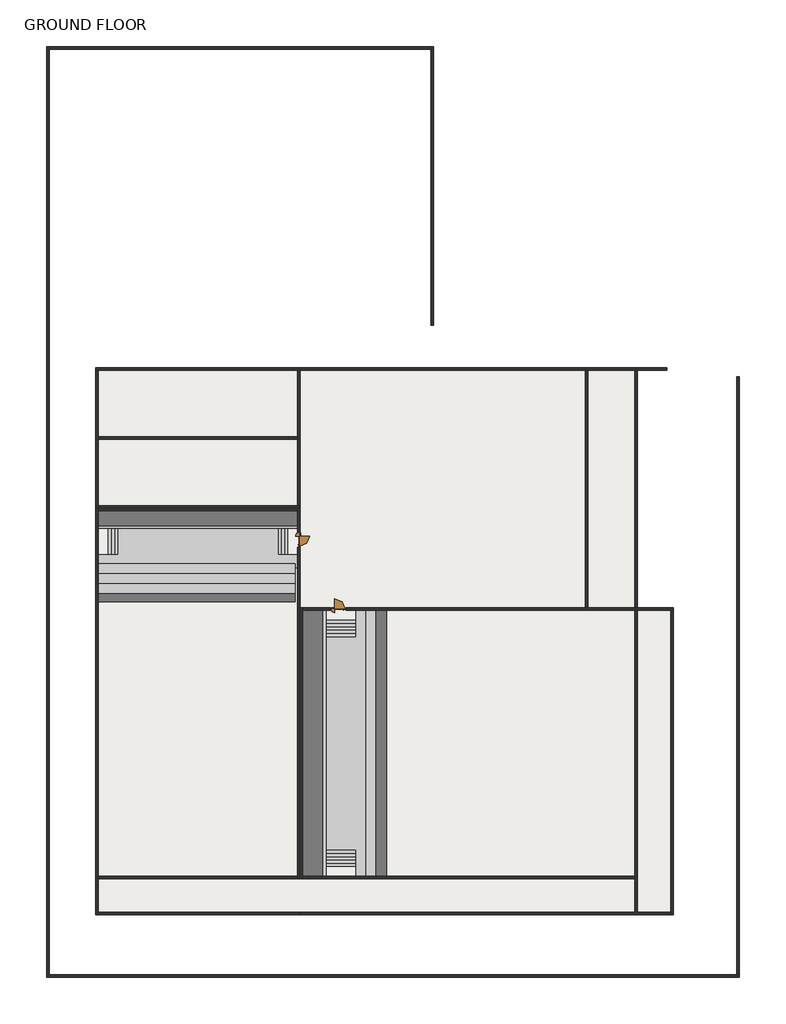
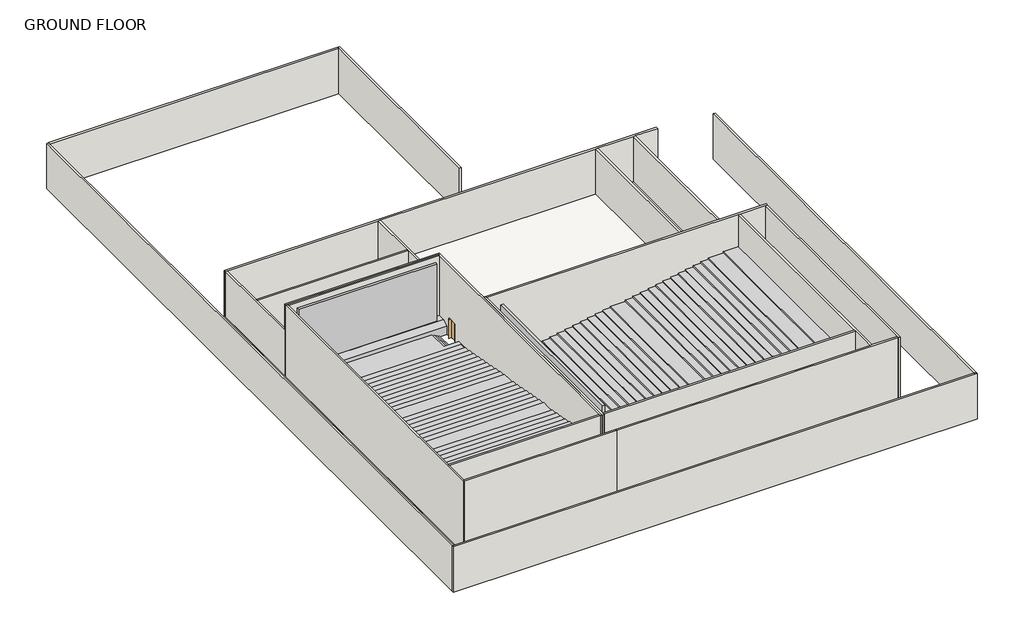
# One storey: 23 walls, 2 doors, 2 stair flights, 1 proxy, 1 slab.
"""IFC4 building model written with IfcOpenShell, lengths in millimetres."""

from ifc_helpers import new_model, si_unit, frame, origin, origin_with_axes, place, context, project, spatial, polyline, outline, extrude, faceted_brep, transform, mapped, element, save
from components import screen_1_screen_1_327eb079, door_1418x2438_e3a65d4f

model = new_model("IFC4")

# Units and contexts
model_context = context("Model", 3, world=origin())
ifc_project = project(units=[si_unit("LENGTHUNIT", "METRE", prefix="MILLI")], contexts=[model_context])

# Site, building, storey
site = spatial("IfcSite", under=ifc_project)
building = spatial("IfcBuilding", under=site)
storey = spatial("IfcBuildingStorey", under=building, Name="GROUND FLOOR", Elevation=0.0)

# Proxy
placement = place(None, origin())
screen_1_screen_1_shape = screen_1_screen_1_327eb079(model_context)
element("IfcBuildingElementProxy", 1, Name="SCREEN 1 : SCREEN 1", ObjectType="SCREEN 1 : SCREEN 1", at=placement, inside=storey, context=model_context, shape_type="MappedRepresentation", body=[
    mapped(screen_1_screen_1_shape, transform((0.0, 0.0, 0.0), x_axis=(1.0, 0.0, 0.0), y_axis=(0.0, 1.0, 0.0), z_axis=(0.0, 0.0, 1.0))),
])

# Doors
door_1418x2438_shape = door_1418x2438_e3a65d4f(model_context)
element("IfcDoor", 2, ObjectType="1418x2438", at=placement, inside=storey, context=model_context, shape_type="MappedRepresentation", body=[
    mapped(door_1418x2438_shape, transform((1375.3587563, 2839.4794445, 0.0), x_axis=(0.0, -1.0, 0.0), y_axis=(1.0, 0.0, 0.0), z_axis=(0.0, 0.0, 1.0))),
])
element("IfcDoor", 3, ObjectType="1418x2438", at=placement, inside=storey, context=model_context, shape_type="MappedRepresentation", body=[
    mapped(door_1418x2438_shape, transform((4956.7587563, -3561.3205555, 0.0), x_axis=(1.0, 0.0, 0.0), y_axis=(0.0, 1.0, 0.0), z_axis=(0.0, 0.0, 1.0))),
])

# Slab
element("IfcSlab", 4, ObjectType="screen room floor 1'", at=placement, inside=storey, context=model_context, shape_type="SweptSolid", body=[
    extrude(outline(polyline([(32426.8587563, 18574.7794445), (32426.8587563, -3447.0205555), (35703.4587563, -3447.0205555), (35703.4587563, -31564.8205555), (-17255.5412437, -31564.8205555), (-17255.5412437, 18574.7794445), (32426.8587563, 18574.7794445)])), frame((0.0, 0.0, -304.8), z_axis=(0.0, 0.0, 1.0), x_axis=(1.0, 0.0, 0.0)), (0.0, 0.0, 1.0), 304.8),
])

# Stair flights
element("IfcStairFlight", 5, ObjectType="3/4\" Nosing", at=placement, inside=storey, context=model_context, shape_type="Brep", body=[
    faceted_brep([(1032.4587563, -322.8205555, 782.5678049), (1032.4587563, 591.5794445, 782.5678049), (-17026.9412437, 591.5794445, 782.5678049), (-17026.9412437, -322.8205555, 782.5678049), (1032.4587563, -322.8205555, 717.941728), (1032.4587563, 249.9315597, 609.6), (1032.4587563, 591.5794445, 609.6), (-17026.9412437, 591.5794445, 609.6), (-17026.9412437, 249.9315597, 609.6), (-17026.9412437, -322.8205555, 717.941728), (1032.4587563, -1237.2205555, 955.5356098), (1032.4587563, -322.8205555, 955.5356098), (-17026.9412437, -322.8205555, 955.5356098), (-17026.9412437, -1237.2205555, 955.5356098), (1032.4587563, -1237.2205555, 890.9095329), (-17026.9412437, -1237.2205555, 890.9095329), (1032.4587563, -2151.6205555, 1128.5034146), (1032.4587563, -1237.2205555, 1128.5034146), (-17026.9412437, -1237.2205555, 1128.5034146), (-17026.9412437, -2151.6205555, 1128.5034146), (1032.4587563, -2151.6205555, 1063.8773378), (-17026.9412437, -2151.6205555, 1063.8773378), (1032.4587563, -3066.0205555, 1301.4712195), (1032.4587563, -2151.6205555, 1301.4712195), (-17026.9412437, -2151.6205555, 1301.4712195), (-17026.9412437, -3066.0205555, 1301.4712195), (1032.4587563, -3066.0205555, 1236.8451427), (-17026.9412437, -3066.0205555, 1236.8451427), (1032.4587563, -3980.4205555, 1474.4390244), (1032.4587563, -3066.0205555, 1474.4390244), (-17026.9412437, -3066.0205555, 1474.4390244), (-17026.9412437, -3980.4205555, 1474.4390244), (1032.4587563, -3980.4205555, 1409.8129475), (-17026.9412437, -3980.4205555, 1409.8129475), (1032.4587563, -4894.8205555, 1647.4068293), (1032.4587563, -3980.4205555, 1647.4068293), (-17026.9412437, -3980.4205555, 1647.4068293), (-17026.9412437, -4894.8205555, 1647.4068293), (1032.4587563, -4894.8205555, 1582.7807524), (-17026.9412437, -4894.8205555, 1582.7807524), (1032.4587563, -5809.2205555, 1820.3746341), (1032.4587563, -4894.8205555, 1820.3746341), (-17026.9412437, -4894.8205555, 1820.3746341), (-17026.9412437, -5809.2205555, 1820.3746341), (1032.4587563, -5809.2205555, 1755.7485573), (-17026.9412437, -5809.2205555, 1755.7485573), (1032.4587563, -6723.6205555, 1993.342439), (1032.4587563, -5809.2205555, 1993.342439), (-17026.9412437, -5809.2205555, 1993.342439), (-17026.9412437, -6723.6205555, 1993.342439), (1032.4587563, -6723.6205555, 1928.7163622), (-17026.9412437, -6723.6205555, 1928.7163622), (1032.4587563, -7638.0205555, 2166.3102439), (1032.4587563, -6723.6205555, 2166.3102439), (-17026.9412437, -6723.6205555, 2166.3102439), (-17026.9412437, -7638.0205555, 2166.3102439), (1032.4587563, -7638.0205555, 2101.684167), (-17026.9412437, -7638.0205555, 2101.684167), (1032.4587563, -8552.4205555, 2512.2458537), (-17026.9412437, -8552.4205555, 2512.2458537), (-17026.9412437, -9472.7735979, 2512.2458537), (-17026.9412437, -10381.2205555, 2512.2458537), (1032.4587563, -10381.2205555, 2512.2458537), (1032.4587563, -9472.7735979, 2512.2458537), (1032.4587563, -8552.4205555, 2339.2780488), (1032.4587563, -10381.2205555, 2448.7458537), (1032.4587563, -9472.7735979, 2448.7458537), (1032.4587563, -8552.4205555, 2274.6519719), (-17026.9412437, -8552.4205555, 2339.2780488), (-17026.9412437, -8552.4205555, 2274.6519719), (-17026.9412437, -9472.7735979, 2448.7458537), (-17026.9412437, -10381.2205555, 2448.7458537), (1032.4587563, -18610.8205555, 4068.9560976), (-17026.9412437, -18610.8205555, 4068.9560976), (-17026.9412437, -18616.7735979, 4068.9560976), (-17026.9412437, -19525.2205555, 4068.9560976), (1032.4587563, -19525.2205555, 4068.9560976), (1032.4587563, -18616.7735979, 4068.9560976), (1032.4587563, -18610.8205555, 3895.9882927), (1032.4587563, -19525.2205555, 4004.3300207), (1032.4587563, -18616.7735979, 3832.4882927), (1032.4587563, -18610.8205555, 3832.4882927), (-17026.9412437, -18610.8205555, 3895.9882927), (-17026.9412437, -18610.8205555, 3832.4882927), (-17026.9412437, -18616.7735979, 3832.4882927), (-17026.9412437, -19525.2205555, 4004.3300207), (1032.4587563, -10387.1735979, 2448.7458537), (-17026.9412437, -10387.1735979, 2448.7458537), (1032.4587563, -11295.6205555, 2620.5875817), (1032.4587563, -12210.0205555, 2793.5553866), (1032.4587563, -13124.4205555, 2966.5231914), (1032.4587563, -14038.8205555, 3139.4909963), (1032.4587563, -14953.2205555, 3312.4588012), (1032.4587563, -15867.6205555, 3485.4266061), (1032.4587563, -16782.0205555, 3658.3944109), (1032.4587563, -17702.3735979, 3832.4882927), (-17026.9412437, -17702.3735979, 3832.4882927), (-17026.9412437, -16782.0205555, 3658.3944109), (-17026.9412437, -15867.6205555, 3485.4266061), (-17026.9412437, -14953.2205555, 3312.4588012), (-17026.9412437, -14038.8205555, 3139.4909963), (-17026.9412437, -13124.4205555, 2966.5231914), (-17026.9412437, -12210.0205555, 2793.5553866), (-17026.9412437, -11295.6205555, 2620.5875817), (1032.4587563, -20439.6205555, 4177.2978256), (1032.4587563, -21354.0205555, 4350.2656305), (1032.4587563, -22268.4205555, 4523.2334353), (1032.4587563, -23182.8205555, 4696.2012402), (1032.4587563, -24097.2205555, 4869.1690451), (1032.4587563, -25011.6205555, 5042.13685), (1032.4587563, -25926.0205555, 5215.1046548), (1032.4587563, -26840.4205555, 5388.0724597), (1032.4587563, -27760.7735979, 5562.1663415), (-17026.9412437, -27760.7735979, 5562.1663415), (-17026.9412437, -26840.4205555, 5388.0724597), (-17026.9412437, -25926.0205555, 5215.1046548), (-17026.9412437, -25011.6205555, 5042.13685), (-17026.9412437, -24097.2205555, 4869.1690451), (-17026.9412437, -23182.8205555, 4696.2012402), (-17026.9412437, -22268.4205555, 4523.2334353), (-17026.9412437, -21354.0205555, 4350.2656305), (-17026.9412437, -20439.6205555, 4177.2978256), (1032.4587563, -7638.0205555, 2339.2780488), (-17026.9412437, -7638.0205555, 2339.2780488), (1032.4587563, -10381.2205555, 2685.2136585), (-17026.9412437, -10381.2205555, 2685.2136585), (-17026.9412437, -10387.1735979, 2685.2136585), (-17026.9412437, -11295.6205555, 2685.2136585), (1032.4587563, -11295.6205555, 2685.2136585), (1032.4587563, -10387.1735979, 2685.2136585), (1032.4587563, -12210.0205555, 2858.1814634), (1032.4587563, -11295.6205555, 2858.1814634), (-17026.9412437, -11295.6205555, 2858.1814634), (-17026.9412437, -12210.0205555, 2858.1814634), (1032.4587563, -13124.4205555, 3031.1492683), (1032.4587563, -12210.0205555, 3031.1492683), (-17026.9412437, -12210.0205555, 3031.1492683), (-17026.9412437, -13124.4205555, 3031.1492683), (1032.4587563, -14038.8205555, 3204.1170732), (1032.4587563, -13124.4205555, 3204.1170732), (-17026.9412437, -13124.4205555, 3204.1170732), (-17026.9412437, -14038.8205555, 3204.1170732), (1032.4587563, -14953.2205555, 3377.084878), (1032.4587563, -14038.8205555, 3377.084878), (-17026.9412437, -14038.8205555, 3377.084878), (-17026.9412437, -14953.2205555, 3377.084878), (1032.4587563, -15867.6205555, 3550.0526829), (1032.4587563, -14953.2205555, 3550.0526829), (-17026.9412437, -14953.2205555, 3550.0526829), (-17026.9412437, -15867.6205555, 3550.0526829), (1032.4587563, -16782.0205555, 3723.0204878), (1032.4587563, -15867.6205555, 3723.0204878), (-17026.9412437, -15867.6205555, 3723.0204878), (-17026.9412437, -16782.0205555, 3723.0204878), (1032.4587563, -16782.0205555, 3895.9882927), (-17026.9412437, -16782.0205555, 3895.9882927), (-17026.9412437, -17702.3735979, 3895.9882927), (1032.4587563, -17702.3735979, 3895.9882927), (1032.4587563, -20439.6205555, 4241.9239024), (1032.4587563, -19525.2205555, 4241.9239024), (-17026.9412437, -19525.2205555, 4241.9239024), (-17026.9412437, -20439.6205555, 4241.9239024), (1032.4587563, -21354.0205555, 4414.8917073), (1032.4587563, -20439.6205555, 4414.8917073), (-17026.9412437, -20439.6205555, 4414.8917073), (-17026.9412437, -21354.0205555, 4414.8917073), (1032.4587563, -22268.4205555, 4587.8595122), (1032.4587563, -21354.0205555, 4587.8595122), (-17026.9412437, -21354.0205555, 4587.8595122), (-17026.9412437, -22268.4205555, 4587.8595122), (1032.4587563, -23182.8205555, 4760.8273171), (1032.4587563, -22268.4205555, 4760.8273171), (-17026.9412437, -22268.4205555, 4760.8273171), (-17026.9412437, -23182.8205555, 4760.8273171), (1032.4587563, -24097.2205555, 4933.795122), (1032.4587563, -23182.8205555, 4933.795122), (-17026.9412437, -23182.8205555, 4933.795122), (-17026.9412437, -24097.2205555, 4933.795122), (1032.4587563, -25011.6205555, 5106.7629268), (1032.4587563, -24097.2205555, 5106.7629268), (-17026.9412437, -24097.2205555, 5106.7629268), (-17026.9412437, -25011.6205555, 5106.7629268), (1032.4587563, -25926.0205555, 5279.7307317), (1032.4587563, -25011.6205555, 5279.7307317), (-17026.9412437, -25011.6205555, 5279.7307317), (-17026.9412437, -25926.0205555, 5279.7307317), (1032.4587563, -26840.4205555, 5452.6985366), (1032.4587563, -25926.0205555, 5452.6985366), (-17026.9412437, -25926.0205555, 5452.6985366), (-17026.9412437, -26840.4205555, 5452.6985366), (1032.4587563, -26840.4205555, 5625.6663415), (-17026.9412437, -26840.4205555, 5625.6663415), (-17026.9412437, -27760.7735979, 5625.6663415), (-17026.9412437, -28059.6205555, 5625.6663415), (1032.4587563, -28059.6205555, 5625.6663415), (1032.4587563, -27760.7735979, 5625.6663415), (1032.4587563, -28059.6205555, 5562.1663415), (-17026.9412437, -28059.6205555, 5562.1663415)], [[[0, 1, 2, 3]], [[1, 0, 4, 5, 6]], [[2, 1, 6, 7]], [[3, 2, 7, 8, 9]], [[10, 11, 12, 13]], [[11, 10, 14, 4, 0]], [[0, 3, 12, 11]], [[13, 12, 3, 9, 15]], [[16, 17, 18, 19]], [[17, 16, 20, 14, 10]], [[10, 13, 18, 17]], [[19, 18, 13, 15, 21]], [[22, 23, 24, 25]], [[23, 22, 26, 20, 16]], [[16, 19, 24, 23]], [[25, 24, 19, 21, 27]], [[28, 29, 30, 31]], [[29, 28, 32, 26, 22]], [[22, 25, 30, 29]], [[31, 30, 25, 27, 33]], [[34, 35, 36, 37]], [[35, 34, 38, 32, 28]], [[28, 31, 36, 35]], [[37, 36, 31, 33, 39]], [[40, 41, 42, 43]], [[41, 40, 44, 38, 34]], [[34, 37, 42, 41]], [[43, 42, 37, 39, 45]], [[46, 47, 48, 49]], [[47, 46, 50, 44, 40]], [[40, 43, 48, 47]], [[49, 48, 43, 45, 51]], [[52, 53, 54, 55]], [[53, 52, 56, 50, 46]], [[46, 49, 54, 53]], [[55, 54, 49, 51, 57]], [[58, 59, 60, 61, 62, 63]], [[64, 58, 63, 62, 65, 66, 67]], [[64, 68, 59, 58]], [[59, 68, 69, 70, 71, 61, 60]], [[72, 73, 74, 75, 76, 77]], [[78, 72, 77, 76, 79, 80, 81]], [[78, 82, 73, 72]], [[73, 82, 83, 84, 85, 75, 74]], [[7, 6, 5, 8]], [[66, 70, 69, 57, 51, 45, 39, 33, 27, 21, 15, 9, 8, 5, 4, 14, 20, 26, 32, 38, 44, 50, 56, 67]], [[70, 66, 65, 86, 87, 71]], [[87, 86, 88, 89, 90, 91, 92, 93, 94, 95, 96, 97, 98, 99, 100, 101, 102, 103]], [[96, 95, 81, 80, 84, 83]], [[84, 80, 79, 104, 105, 106, 107, 108, 109, 110, 111, 112, 113, 114, 115, 116, 117, 118, 119, 120, 121, 85]], [[64, 122, 123, 68]], [[122, 64, 67, 56, 52]], [[52, 55, 123, 122]], [[68, 123, 55, 57, 69]], [[124, 125, 126, 127, 128, 129]], [[62, 124, 129, 128, 88, 86, 65]], [[62, 61, 125, 124]], [[125, 61, 71, 87, 103, 127, 126]], [[130, 131, 132, 133]], [[131, 130, 89, 88, 128]], [[128, 127, 132, 131]], [[133, 132, 127, 103, 102]], [[134, 135, 136, 137]], [[135, 134, 90, 89, 130]], [[130, 133, 136, 135]], [[137, 136, 133, 102, 101]], [[138, 139, 140, 141]], [[139, 138, 91, 90, 134]], [[134, 137, 140, 139]], [[141, 140, 137, 101, 100]], [[142, 143, 144, 145]], [[143, 142, 92, 91, 138]], [[138, 141, 144, 143]], [[145, 144, 141, 100, 99]], [[146, 147, 148, 149]], [[147, 146, 93, 92, 142]], [[142, 145, 148, 147]], [[149, 148, 145, 99, 98]], [[150, 151, 152, 153]], [[151, 150, 94, 93, 146]], [[146, 149, 152, 151]], [[153, 152, 149, 98, 97]], [[154, 155, 156, 82, 78, 157]], [[150, 154, 157, 78, 81, 95, 94]], [[150, 153, 155, 154]], [[155, 153, 97, 96, 83, 82, 156]], [[158, 159, 160, 161]], [[159, 158, 104, 79, 76]], [[76, 75, 160, 159]], [[161, 160, 75, 85, 121]], [[162, 163, 164, 165]], [[163, 162, 105, 104, 158]], [[158, 161, 164, 163]], [[165, 164, 161, 121, 120]], [[166, 167, 168, 169]], [[167, 166, 106, 105, 162]], [[162, 165, 168, 167]], [[169, 168, 165, 120, 119]], [[170, 171, 172, 173]], [[171, 170, 107, 106, 166]], [[166, 169, 172, 171]], [[173, 172, 169, 119, 118]], [[174, 175, 176, 177]], [[175, 174, 108, 107, 170]], [[170, 173, 176, 175]], [[177, 176, 173, 118, 117]], [[178, 179, 180, 181]], [[179, 178, 109, 108, 174]], [[174, 177, 180, 179]], [[181, 180, 177, 117, 116]], [[182, 183, 184, 185]], [[183, 182, 110, 109, 178]], [[178, 181, 184, 183]], [[185, 184, 181, 116, 115]], [[186, 187, 188, 189]], [[187, 186, 111, 110, 182]], [[182, 185, 188, 187]], [[189, 188, 185, 115, 114]], [[190, 191, 192, 193, 194, 195]], [[186, 190, 195, 194, 196, 112, 111]], [[186, 189, 191, 190]], [[191, 189, 114, 113, 197, 193, 192]], [[194, 193, 197, 196]], [[113, 112, 196, 197]]]),
])
element("IfcStairFlight", 6, ObjectType="3/4\" Nosing", at=placement, inside=storey, context=model_context, shape_type="Brep", body=[
    faceted_brep([(8423.8587563, -3675.6205555, 1085.3853659), (7509.4587563, -3675.6205555, 1085.3853659), (7509.4587563, -28059.6205555, 1085.3853659), (8423.8587563, -28059.6205555, 1085.3853659), (8423.8587563, -3675.6205555, 1020.7847351), (7854.9316945, -3675.6205555, 914.4), (7509.4587563, -3675.6205555, 914.4), (7509.4587563, -28059.6205555, 914.4), (7854.9316945, -28059.6205555, 914.4), (8423.8587563, -28059.6205555, 1020.7847351), (9338.2587563, -3675.6205555, 1256.3707317), (8423.8587563, -3675.6205555, 1256.3707317), (8423.8587563, -28059.6205555, 1256.3707317), (9338.2587563, -28059.6205555, 1256.3707317), (9338.2587563, -3675.6205555, 1191.770101), (9338.2587563, -28059.6205555, 1191.770101), (10252.6587563, -3675.6205555, 1427.3560976), (9338.2587563, -3675.6205555, 1427.3560976), (9338.2587563, -28059.6205555, 1427.3560976), (10252.6587563, -28059.6205555, 1427.3560976), (10252.6587563, -3675.6205555, 1362.7554668), (10252.6587563, -28059.6205555, 1362.7554668), (11167.0587563, -3675.6205555, 1598.3414634), (10252.6587563, -3675.6205555, 1598.3414634), (10252.6587563, -28059.6205555, 1598.3414634), (11167.0587563, -28059.6205555, 1598.3414634), (11167.0587563, -3675.6205555, 1533.7408327), (11167.0587563, -28059.6205555, 1533.7408327), (12081.4587563, -3675.6205555, 1769.3268293), (11167.0587563, -3675.6205555, 1769.3268293), (11167.0587563, -28059.6205555, 1769.3268293), (12081.4587563, -28059.6205555, 1769.3268293), (12081.4587563, -3675.6205555, 1704.7261985), (12081.4587563, -28059.6205555, 1704.7261985), (12995.8587563, -3675.6205555, 1940.3121951), (12081.4587563, -3675.6205555, 1940.3121951), (12081.4587563, -28059.6205555, 1940.3121951), (12995.8587563, -28059.6205555, 1940.3121951), (12995.8587563, -3675.6205555, 1875.7115644), (12995.8587563, -28059.6205555, 1875.7115644), (13910.2587563, -3675.6205555, 2111.297561), (12995.8587563, -3675.6205555, 2111.297561), (12995.8587563, -28059.6205555, 2111.297561), (13910.2587563, -28059.6205555, 2111.297561), (13910.2587563, -3675.6205555, 2046.6969303), (13910.2587563, -28059.6205555, 2046.6969303), (14824.6587563, -3675.6205555, 2282.2829268), (13910.2587563, -3675.6205555, 2282.2829268), (13910.2587563, -28059.6205555, 2282.2829268), (14824.6587563, -28059.6205555, 2282.2829268), (14824.6587563, -3675.6205555, 2217.6822961), (14824.6587563, -28059.6205555, 2217.6822961), (15739.0587563, -3675.6205555, 2453.2682927), (14824.6587563, -3675.6205555, 2453.2682927), (14824.6587563, -28059.6205555, 2453.2682927), (15739.0587563, -28059.6205555, 2453.2682927), (15739.0587563, -3675.6205555, 2388.667662), (15739.0587563, -28059.6205555, 2388.667662), (16653.4587563, -3675.6205555, 2624.2536585), (15739.0587563, -3675.6205555, 2624.2536585), (15739.0587563, -28059.6205555, 2624.2536585), (16653.4587563, -28059.6205555, 2624.2536585), (16653.4587563, -3675.6205555, 2559.6530278), (16653.4587563, -28059.6205555, 2559.6530278), (16653.4587563, -3675.6205555, 2795.2390244), (16653.4587563, -28059.6205555, 2795.2390244), (17573.7447379, -28059.6205555, 2795.2390244), (18482.2587563, -28059.6205555, 2795.2390244), (18482.2587563, -3675.6205555, 2795.2390244), (17573.7447379, -3675.6205555, 2795.2390244), (18482.2587563, -3675.6205555, 2731.7390244), (17573.7447379, -3675.6205555, 2731.7390244), (17573.7447379, -28059.6205555, 2731.7390244), (18482.2587563, -28059.6205555, 2731.7390244), (18482.2587563, -3675.6205555, 2966.2243902), (18482.2587563, -28059.6205555, 2966.2243902), (18488.1447379, -28059.6205555, 2966.2243902), (19396.6587563, -28059.6205555, 2966.2243902), (19396.6587563, -3675.6205555, 2966.2243902), (18488.1447379, -3675.6205555, 2966.2243902), (19396.6587563, -3675.6205555, 2901.6237595), (18488.1447379, -3675.6205555, 2731.7390244), (18488.1447379, -28059.6205555, 2731.7390244), (19396.6587563, -28059.6205555, 2901.6237595), (20311.0587563, -3675.6205555, 3137.2097561), (19396.6587563, -3675.6205555, 3137.2097561), (19396.6587563, -28059.6205555, 3137.2097561), (20311.0587563, -28059.6205555, 3137.2097561), (20311.0587563, -3675.6205555, 3072.6091254), (20311.0587563, -28059.6205555, 3072.6091254), (21225.4587563, -3675.6205555, 3308.195122), (20311.0587563, -3675.6205555, 3308.195122), (20311.0587563, -28059.6205555, 3308.195122), (21225.4587563, -28059.6205555, 3308.195122), (21225.4587563, -3675.6205555, 3243.5944912), (21225.4587563, -28059.6205555, 3243.5944912), (22139.8587563, -3675.6205555, 3479.1804878), (21225.4587563, -3675.6205555, 3479.1804878), (21225.4587563, -28059.6205555, 3479.1804878), (22139.8587563, -28059.6205555, 3479.1804878), (22139.8587563, -3675.6205555, 3414.5798571), (22139.8587563, -28059.6205555, 3414.5798571), (23054.2587563, -3675.6205555, 3650.1658537), (22139.8587563, -3675.6205555, 3650.1658537), (22139.8587563, -28059.6205555, 3650.1658537), (23054.2587563, -28059.6205555, 3650.1658537), (23054.2587563, -3675.6205555, 3585.5652229), (23054.2587563, -28059.6205555, 3585.5652229), (23968.6587563, -3675.6205555, 3821.1512195), (23054.2587563, -3675.6205555, 3821.1512195), (23054.2587563, -28059.6205555, 3821.1512195), (23968.6587563, -28059.6205555, 3821.1512195), (23968.6587563, -3675.6205555, 3756.5505888), (23968.6587563, -28059.6205555, 3756.5505888), (24883.0587563, -3675.6205555, 3992.1365854), (23968.6587563, -3675.6205555, 3992.1365854), (23968.6587563, -28059.6205555, 3992.1365854), (24883.0587563, -28059.6205555, 3992.1365854), (24883.0587563, -3675.6205555, 3927.5359546), (24883.0587563, -28059.6205555, 3927.5359546), (25797.4587563, -3675.6205555, 4163.1219512), (24883.0587563, -3675.6205555, 4163.1219512), (24883.0587563, -28059.6205555, 4163.1219512), (25797.4587563, -28059.6205555, 4163.1219512), (25797.4587563, -3675.6205555, 4098.5213205), (25797.4587563, -28059.6205555, 4098.5213205), (26711.8587563, -3675.6205555, 4334.1073171), (25797.4587563, -3675.6205555, 4334.1073171), (25797.4587563, -28059.6205555, 4334.1073171), (26711.8587563, -28059.6205555, 4334.1073171), (26711.8587563, -3675.6205555, 4269.5066863), (26711.8587563, -28059.6205555, 4269.5066863), (27626.2587563, -3675.6205555, 4505.0926829), (26711.8587563, -3675.6205555, 4505.0926829), (26711.8587563, -28059.6205555, 4505.0926829), (27626.2587563, -28059.6205555, 4505.0926829), (27626.2587563, -3675.6205555, 4440.4920522), (27626.2587563, -28059.6205555, 4440.4920522), (28540.6587563, -3675.6205555, 4676.0780488), (27626.2587563, -3675.6205555, 4676.0780488), (27626.2587563, -28059.6205555, 4676.0780488), (28540.6587563, -28059.6205555, 4676.0780488), (28540.6587563, -3675.6205555, 4612.3011104), (28540.6587563, -3675.6205555, 4611.4774181), (28540.6587563, -28059.6205555, 4611.4774181), (28540.6587563, -28059.6205555, 4612.3011104), (30369.4587563, -3675.6205555, 4847.0634146), (28540.6587563, -3675.6205555, 4847.0634146), (28540.6587563, -28059.6205555, 4847.0634146), (30369.4587563, -28059.6205555, 4847.0634146), (30369.4587563, -3675.6205555, 4783.2864762), (30369.4587563, -28059.6205555, 4783.2864762), (32198.2587563, -3675.6205555, 4954.2718421), (32198.2587563, -28059.6205555, 4954.2718421), (32198.2587563, -3675.6205555, 5018.0487805), (30369.4587563, -3675.6205555, 5018.0487805), (30369.4587563, -28059.6205555, 5018.0487805), (32198.2587563, -28059.6205555, 5018.0487805)], [[[0, 1, 2, 3]], [[1, 0, 4, 5, 6]], [[2, 1, 6, 7]], [[3, 2, 7, 8, 9]], [[10, 11, 12, 13]], [[11, 10, 14, 4, 0]], [[0, 3, 12, 11]], [[13, 12, 3, 9, 15]], [[16, 17, 18, 19]], [[17, 16, 20, 14, 10]], [[10, 13, 18, 17]], [[19, 18, 13, 15, 21]], [[22, 23, 24, 25]], [[23, 22, 26, 20, 16]], [[16, 19, 24, 23]], [[25, 24, 19, 21, 27]], [[28, 29, 30, 31]], [[29, 28, 32, 26, 22]], [[22, 25, 30, 29]], [[31, 30, 25, 27, 33]], [[34, 35, 36, 37]], [[35, 34, 38, 32, 28]], [[28, 31, 36, 35]], [[37, 36, 31, 33, 39]], [[40, 41, 42, 43]], [[41, 40, 44, 38, 34]], [[34, 37, 42, 41]], [[43, 42, 37, 39, 45]], [[46, 47, 48, 49]], [[47, 46, 50, 44, 40]], [[40, 43, 48, 47]], [[49, 48, 43, 45, 51]], [[52, 53, 54, 55]], [[53, 52, 56, 50, 46]], [[46, 49, 54, 53]], [[55, 54, 49, 51, 57]], [[58, 59, 60, 61]], [[59, 58, 62, 56, 52]], [[52, 55, 60, 59]], [[61, 60, 55, 57, 63]], [[64, 65, 66, 67, 68, 69]], [[58, 64, 69, 68, 70, 71, 62]], [[58, 61, 65, 64]], [[65, 61, 63, 72, 73, 67, 66]], [[74, 75, 76, 77, 78, 79]], [[68, 74, 79, 78, 80, 81, 70]], [[68, 67, 75, 74]], [[75, 67, 73, 82, 83, 77, 76]], [[84, 85, 86, 87]], [[85, 84, 88, 80, 78]], [[78, 77, 86, 85]], [[87, 86, 77, 83, 89]], [[90, 91, 92, 93]], [[91, 90, 94, 88, 84]], [[84, 87, 92, 91]], [[93, 92, 87, 89, 95]], [[96, 97, 98, 99]], [[97, 96, 100, 94, 90]], [[90, 93, 98, 97]], [[99, 98, 93, 95, 101]], [[102, 103, 104, 105]], [[103, 102, 106, 100, 96]], [[96, 99, 104, 103]], [[105, 104, 99, 101, 107]], [[108, 109, 110, 111]], [[109, 108, 112, 106, 102]], [[102, 105, 110, 109]], [[111, 110, 105, 107, 113]], [[114, 115, 116, 117]], [[115, 114, 118, 112, 108]], [[108, 111, 116, 115]], [[117, 116, 111, 113, 119]], [[120, 121, 122, 123]], [[121, 120, 124, 118, 114]], [[114, 117, 122, 121]], [[123, 122, 117, 119, 125]], [[126, 127, 128, 129]], [[127, 126, 130, 124, 120]], [[120, 123, 128, 127]], [[129, 128, 123, 125, 131]], [[132, 133, 134, 135]], [[133, 132, 136, 130, 126]], [[126, 129, 134, 133]], [[135, 134, 129, 131, 137]], [[138, 139, 140, 141]], [[139, 138, 142, 143, 136, 132]], [[132, 135, 140, 139]], [[141, 140, 135, 137, 144, 145]], [[146, 147, 148, 149]], [[147, 146, 150, 142, 138]], [[138, 141, 148, 147]], [[149, 148, 141, 145, 151]], [[7, 6, 5, 8]], [[71, 72, 63, 57, 51, 45, 39, 33, 27, 21, 15, 9, 8, 5, 4, 14, 20, 26, 32, 38, 44, 50, 56, 62]], [[72, 71, 70, 81, 82, 73]], [[143, 144, 137, 131, 125, 119, 113, 107, 101, 95, 89, 83, 82, 81, 80, 88, 94, 100, 106, 112, 118, 124, 130, 136]], [[144, 143, 142, 145]], [[145, 142, 150, 152, 153, 151]], [[154, 155, 156, 157]], [[155, 154, 152, 150, 146]], [[146, 149, 156, 155]], [[157, 156, 149, 151, 153]], [[154, 157, 153, 152]]]),
])

# Walls
element("IfcWall", 7, ObjectType="9\" inch wall", at=placement, inside=storey, context=model_context, shape_type="Brep", body=[
    faceted_brep([(-17255.5412437, 5696.9794445, 9144.0), (-17255.5412437, 5696.9794445, 0.0), (-17255.5412437, -31564.8205555, 0.0), (-17255.5412437, -31564.8205555, 9144.0), (-17026.9412437, 5696.9794445, 0.0), (-17026.9412437, 5696.9794445, 9144.0), (-17026.9412437, 5468.3794445, 9144.0), (-17026.9412437, -28059.6205555, 9144.0), (-17026.9412437, -28288.2205555, 9144.0), (-17026.9412437, -31336.2205555, 9144.0), (-17026.9412437, -31564.8205555, 9144.0), (-17026.9412437, -31564.8205555, 0.0), (-17026.9412437, -31336.2205555, 0.0), (-17026.9412437, -28288.2205555, 0.0), (-17026.9412437, -28059.6205555, 0.0), (-17026.9412437, 5468.3794445, 0.0)], [[[0, 1, 2, 3]], [[4, 5, 6, 7, 8, 9, 10, 11, 12, 13, 14, 15]], [[2, 1, 4, 15, 14, 13, 12, 11]], [[0, 3, 10, 9, 8, 7, 6, 5]], [[3, 2, 11, 10]], [[0, 5, 4, 1]]]),
])
element("IfcWall", 8, ObjectType="9\" inch wall", at=placement, inside=storey, context=model_context, shape_type="SweptSolid", body=[
    extrude(outline(polyline([(1375.3587563, -31564.8205555), (-17026.9412437, -31564.8205555), (-17026.9412437, -31336.2205555), (1375.3587563, -31336.2205555), (1375.3587563, -31564.8205555)])), origin_with_axes(), (0.0, 0.0, 1.0), 9144.0),
])
element("IfcWall", 9, ObjectType="9\" inch wall", at=placement, inside=storey, context=model_context, shape_type="Brep", body=[
    faceted_brep([(1489.6587563, 5696.9794445, 9144.0), (1489.6587563, -28288.2205555, 9144.0), (1489.6587563, -28288.2205555, 0.0), (1489.6587563, 2130.7294445, 0.0), (1489.6587563, 2130.7294445, 2438.4), (1489.6587563, 3548.2294445, 2438.4), (1489.6587563, 3548.2294445, 0.0), (1489.6587563, 5696.9794445, 0.0), (1261.0587563, -28288.2205555, 9144.0), (1261.0587563, -28059.6205555, 9144.0), (1261.0587563, 5468.3794445, 9144.0), (1261.0587563, 5696.9794445, 9144.0), (1261.0587563, 5696.9794445, 0.0), (1261.0587563, 5468.3794445, 0.0), (1261.0587563, 3548.2294445, 0.0), (1261.0587563, 3548.2294445, 2438.4), (1261.0587563, 2130.7294445, 2438.4), (1261.0587563, 2130.7294445, 0.0), (1261.0587563, -28059.6205555, 0.0), (1261.0587563, -28288.2205555, 0.0), (1392.6587563, 2130.7294445, 0.0), (1392.6587563, 2115.7294445, 0.0), (1469.6587563, 2115.7294445, 0.0), (1469.6587563, 2130.7294445, 0.0), (1469.6587563, 3548.2294445, 0.0), (1469.6587563, 3563.2294445, 0.0), (1392.6587563, 3563.2294445, 0.0), (1392.6587563, 3548.2294445, 0.0), (1469.6587563, 2130.7294445, 2438.4), (1469.6587563, 3548.2294445, 2438.4), (1469.6587563, 2115.7294445, 2453.4), (1469.6587563, 3563.2294445, 2453.4), (1392.6587563, 2115.7294445, 2453.4), (1392.6587563, 2130.7294445, 2438.4), (1392.6587563, 3548.2294445, 2438.4), (1392.6587563, 3563.2294445, 2453.4)], [[[0, 1, 2, 3, 4, 5, 6, 7]], [[8, 9, 10, 11, 12, 13, 14, 15, 16, 17, 18, 19]], [[2, 19, 18, 17, 20, 21, 22, 23, 3]], [[12, 7, 6, 24, 25, 26, 27, 14, 13]], [[1, 0, 11, 10, 9, 8]], [[2, 1, 8, 19]], [[7, 12, 11, 0]], [[23, 28, 4, 3]], [[29, 24, 6, 5]], [[28, 29, 5, 4]], [[28, 23, 22, 30, 31, 25, 24, 29]], [[30, 22, 21, 32]], [[32, 21, 20, 33, 34, 27, 26, 35]], [[31, 30, 32, 35]], [[25, 31, 35, 26]], [[33, 20, 17, 16]], [[27, 34, 15, 14]], [[34, 33, 16, 15]]]),
])
element("IfcWall", 10, ObjectType="9\" inch wall", at=placement, inside=storey, context=model_context, shape_type="Brep", body=[
    faceted_brep([(1718.2587563, -28288.2205555, 0.0), (1718.2587563, -28059.6205555, 0.0), (1718.2587563, -3675.6205555, 0.0), (1718.2587563, -3447.0205555, 0.0), (1718.2587563, -3447.0205555, 9144.0), (1718.2587563, -3675.6205555, 9144.0), (1718.2587563, -28059.6205555, 9144.0), (1718.2587563, -28288.2205555, 9144.0), (1489.6587563, -28288.2205555, 0.0), (1489.6587563, -28288.2205555, 9144.0), (1489.6587563, -3447.0205555, 9144.0), (1489.6587563, -3447.0205555, 0.0)], [[[0, 1, 2, 3, 4, 5, 6, 7]], [[8, 9, 10, 11]], [[3, 2, 1, 0, 8, 11]], [[7, 6, 5, 4, 10, 9]], [[4, 3, 11, 10]], [[0, 7, 9, 8]]]),
])
element("IfcWall", 11, ObjectType="9\" inch wall", at=placement, inside=storey, context=model_context, shape_type="Brep", body=[
    faceted_brep([(35703.4587563, -3675.6205555, 9144.0), (35474.8587563, -3675.6205555, 9144.0), (32426.8587563, -3675.6205555, 9144.0), (32198.2587563, -3675.6205555, 9144.0), (1718.2587563, -3675.6205555, 9144.0), (1718.2587563, -3675.6205555, 0.0), (4248.0087563, -3675.6205555, 0.0), (4248.0087563, -3675.6205555, 2438.4), (5665.5087563, -3675.6205555, 2438.4), (5665.5087563, -3675.6205555, 0.0), (32198.2587563, -3675.6205555, 0.0), (32426.8587563, -3675.6205555, 0.0), (35474.8587563, -3675.6205555, 0.0), (35703.4587563, -3675.6205555, 0.0), (1718.2587563, -3447.0205555, 9144.0), (35703.4587563, -3447.0205555, 9144.0), (35703.4587563, -3447.0205555, 0.0), (32426.8587563, -3447.0205555, 0.0), (32198.2587563, -3447.0205555, 0.0), (27854.8587563, -3447.0205555, 0.0), (27626.2587563, -3447.0205555, 0.0), (5665.5087563, -3447.0205555, 0.0), (5665.5087563, -3447.0205555, 2438.4), (4248.0087563, -3447.0205555, 2438.4), (4248.0087563, -3447.0205555, 0.0), (1718.2587563, -3447.0205555, 0.0), (4248.0087563, -3467.0205555, 0.0), (4233.0087563, -3467.0205555, 0.0), (4233.0087563, -3544.0205555, 0.0), (4248.0087563, -3544.0205555, 0.0), (5665.5087563, -3544.0205555, 0.0), (5680.5087563, -3544.0205555, 0.0), (5680.5087563, -3467.0205555, 0.0), (5665.5087563, -3467.0205555, 0.0), (5665.5087563, -3467.0205555, 2438.4), (4248.0087563, -3467.0205555, 2438.4), (5680.5087563, -3467.0205555, 2453.4), (4233.0087563, -3467.0205555, 2453.4), (5680.5087563, -3544.0205555, 2453.4), (5665.5087563, -3544.0205555, 2438.4), (4248.0087563, -3544.0205555, 2438.4), (4233.0087563, -3544.0205555, 2453.4)], [[[0, 1, 2, 3, 4, 5, 6, 7, 8, 9, 10, 11, 12, 13]], [[14, 15, 16, 17, 18, 19, 20, 21, 22, 23, 24, 25]], [[5, 25, 24, 26, 27, 28, 29, 6]], [[16, 13, 12, 11, 10, 9, 30, 31, 32, 33, 21, 20, 19, 18, 17]], [[4, 3, 2, 1, 0, 15, 14]], [[5, 4, 14, 25]], [[0, 13, 16, 15]], [[33, 34, 22, 21]], [[35, 26, 24, 23]], [[34, 35, 23, 22]], [[34, 33, 32, 36, 37, 27, 26, 35]], [[36, 32, 31, 38]], [[38, 31, 30, 39, 40, 29, 28, 41]], [[37, 36, 38, 41]], [[27, 37, 41, 28]], [[39, 30, 9, 8]], [[29, 40, 7, 6]], [[40, 39, 8, 7]]]),
])
element("IfcWall", 12, ObjectType="9\" inch wall", at=placement, inside=storey, context=model_context, shape_type="Brep", body=[
    faceted_brep([(35474.8587563, -3675.6205555, 0.0), (35474.8587563, -31336.2205555, 0.0), (35474.8587563, -31564.8205555, 0.0), (35474.8587563, -31564.8205555, 9144.0), (35474.8587563, -31336.2205555, 9144.0), (35474.8587563, -3675.6205555, 9144.0), (35703.4587563, -3675.6205555, 0.0), (35703.4587563, -3675.6205555, 9144.0), (35703.4587563, -31564.8205555, 9144.0), (35703.4587563, -31564.8205555, 0.0)], [[[0, 1, 2, 3, 4, 5]], [[6, 7, 8, 9]], [[2, 1, 0, 6, 9]], [[5, 4, 3, 8, 7]], [[0, 5, 7, 6]], [[3, 2, 9, 8]]]),
])
element("IfcWall", 13, ObjectType="9\" inch wall", at=placement, inside=storey, context=model_context, shape_type="Brep", body=[
    faceted_brep([(35474.8587563, -31336.2205555, 0.0), (32426.8587563, -31336.2205555, 0.0), (32198.2587563, -31336.2205555, 0.0), (1375.3587563, -31336.2205555, 0.0), (1375.3587563, -31336.2205555, 9144.0), (32198.2587563, -31336.2205555, 9144.0), (32426.8587563, -31336.2205555, 9144.0), (35474.8587563, -31336.2205555, 9144.0), (35474.8587563, -31564.8205555, 0.0), (35474.8587563, -31564.8205555, 9144.0), (1375.3587563, -31564.8205555, 9144.0), (1375.3587563, -31564.8205555, 0.0)], [[[0, 1, 2, 3, 4, 5, 6, 7]], [[8, 9, 10, 11]], [[3, 2, 1, 0, 8, 11]], [[4, 3, 11, 10]], [[7, 6, 5, 4, 10, 9]], [[0, 7, 9, 8]]]),
])
element("IfcWall", 14, ObjectType="9\" inch wall", at=placement, inside=storey, context=model_context, shape_type="Brep", body=[
    faceted_brep([(-17255.5412437, 18346.1794445, 0.0), (-17026.9412437, 18346.1794445, 0.0), (1261.0587563, 18346.1794445, 0.0), (1489.6587563, 18346.1794445, 0.0), (27626.2587563, 18346.1794445, 0.0), (27854.8587563, 18346.1794445, 0.0), (32198.2587563, 18346.1794445, 0.0), (32426.8587563, 18346.1794445, 0.0), (35131.9587563, 18346.1794445, 0.0), (35131.9587563, 18346.1794445, 5798.6341463), (32426.8587563, 18346.1794445, 5798.6341463), (32198.2587563, 18346.1794445, 5798.6341463), (27854.8587563, 18346.1794445, 5798.6341463), (27626.2587563, 18346.1794445, 5798.6341463), (1489.6587563, 18346.1794445, 5798.6341463), (1261.0587563, 18346.1794445, 5798.6341463), (-17026.9412437, 18346.1794445, 5798.6341463), (-17255.5412437, 18346.1794445, 5798.6341463), (-17255.5412437, 18574.7794445, 0.0), (-17255.5412437, 18574.7794445, 5798.6341463), (35131.9587563, 18574.7794445, 5798.6341463), (35131.9587563, 18574.7794445, 0.0)], [[[0, 1, 2, 3, 4, 5, 6, 7, 8, 9, 10, 11, 12, 13, 14, 15, 16, 17]], [[18, 19, 20, 21]], [[8, 7, 6, 5, 4, 3, 2, 1, 0, 18, 21]], [[9, 8, 21, 20]], [[17, 16, 15, 14, 13, 12, 11, 10, 9, 20, 19]], [[0, 17, 19, 18]]]),
])
element("IfcWall", 15, ObjectType="9\" inch wall", at=placement, inside=storey, context=model_context, shape_type="Brep", body=[
    faceted_brep([(41761.3587563, -37089.3205555, 0.0), (41532.7587563, -37089.3205555, 0.0), (-21560.8412437, -37089.3205555, 0.0), (-21789.4412437, -37089.3205555, 0.0), (-21789.4412437, -37089.3205555, 5798.6341463), (-21560.8412437, -37089.3205555, 5798.6341463), (41532.7587563, -37089.3205555, 5798.6341463), (41761.3587563, -37089.3205555, 5798.6341463), (41761.3587563, -37317.9205555, 0.0), (41761.3587563, -37317.9205555, 5798.6341463), (-21789.4412437, -37317.9205555, 5798.6341463), (-21789.4412437, -37317.9205555, 0.0)], [[[0, 1, 2, 3, 4, 5, 6, 7]], [[8, 9, 10, 11]], [[3, 2, 1, 0, 8, 11]], [[7, 6, 5, 4, 10, 9]], [[4, 3, 11, 10]], [[0, 7, 9, 8]]]),
])
element("IfcWall", 16, ObjectType="9\" inch wall", at=placement, inside=storey, context=model_context, shape_type="Brep", body=[
    faceted_brep([(-21560.8412437, -37089.3205555, 0.0), (-21560.8412437, 47797.4794445, 0.0), (-21560.8412437, 48026.0794445, 0.0), (-21560.8412437, 48026.0794445, 5798.6341463), (-21560.8412437, 47797.4794445, 5798.6341463), (-21560.8412437, -37089.3205555, 5798.6341463), (-21789.4412437, -37089.3205555, 0.0), (-21789.4412437, -37089.3205555, 5798.6341463), (-21789.4412437, 48026.0794445, 5798.6341463), (-21789.4412437, 48026.0794445, 0.0)], [[[0, 1, 2, 3, 4, 5]], [[6, 7, 8, 9]], [[2, 1, 0, 6, 9]], [[5, 4, 3, 8, 7]], [[0, 5, 7, 6]], [[3, 2, 9, 8]]]),
])
element("IfcWall", 17, ObjectType="9\" inch wall", at=placement, inside=storey, context=model_context, shape_type="SweptSolid", body=[
    extrude(outline(polyline([(13491.1587563, 47797.4794445), (-21560.8412437, 47797.4794445), (-21560.8412437, 48026.0794445), (13491.1587563, 48026.0794445), (13491.1587563, 47797.4794445)])), origin_with_axes(), (0.0, 0.0, 1.0), 5798.6341463),
])
element("IfcWall", 18, ObjectType="9\" inch wall", at=placement, inside=storey, context=model_context, shape_type="Brep", body=[
    faceted_brep([(13719.7587563, 22460.9794445, 0.0), (13719.7587563, 48026.0794445, 0.0), (13719.7587563, 48026.0794445, 5798.6341463), (13719.7587563, 22460.9794445, 5798.6341463), (13491.1587563, 22460.9794445, 0.0), (13491.1587563, 22460.9794445, 5798.6341463), (13491.1587563, 47797.4794445, 5798.6341463), (13491.1587563, 48026.0794445, 5798.6341463), (13491.1587563, 48026.0794445, 0.0), (13491.1587563, 47797.4794445, 0.0)], [[[0, 1, 2, 3]], [[4, 5, 6, 7, 8, 9]], [[1, 0, 4, 9, 8]], [[3, 2, 7, 6, 5]], [[0, 3, 5, 4]], [[2, 1, 8, 7]]]),
])
element("IfcWall", 19, ObjectType="9\" inch wall", at=placement, inside=storey, context=model_context, shape_type="SweptSolid", body=[
    extrude(outline(polyline([(41532.7587563, -37089.3205555), (41532.7587563, 17736.5794445), (41761.3587563, 17736.5794445), (41761.3587563, -37089.3205555), (41532.7587563, -37089.3205555)])), origin_with_axes(), (0.0, 0.0, 1.0), 5798.6341463),
])
element("IfcWall", 20, ObjectType="9\" inch wall", at=placement, inside=storey, context=model_context, shape_type="SweptSolid", body=[
    extrude(outline(polyline([(27626.2587563, -3447.0205555), (27626.2587563, 18346.1794445), (27854.8587563, 18346.1794445), (27854.8587563, -3447.0205555), (27626.2587563, -3447.0205555)])), origin_with_axes(), (0.0, 0.0, 1.0), 5798.6341463),
])
element("IfcWall", 21, ObjectType="9\" inch wall", at=placement, inside=storey, context=model_context, shape_type="SweptSolid", body=[
    extrude(outline(polyline([(32426.8587563, 18346.1794445), (32426.8587563, -3447.0205555), (32198.2587563, -3447.0205555), (32198.2587563, 18346.1794445), (32426.8587563, 18346.1794445)])), origin_with_axes(), (0.0, 0.0, 1.0), 5798.6341463),
])
element("IfcWall", 22, ObjectType="9\" inch wall", at=placement, inside=storey, context=model_context, shape_type="SweptSolid", body=[
    extrude(outline(polyline([(1261.0587563, 5468.3794445), (-17026.9412437, 5468.3794445), (-17026.9412437, 5696.9794445), (1261.0587563, 5696.9794445), (1261.0587563, 5468.3794445)])), origin_with_axes(), (0.0, 0.0, 1.0), 9144.0),
])
element("IfcWall", 23, ObjectType="9\" inch wall", at=placement, inside=storey, context=model_context, shape_type="SweptSolid", body=[
    extrude(outline(polyline([(1261.0587563, -28288.2205555), (-17026.9412437, -28288.2205555), (-17026.9412437, -28059.6205555), (1261.0587563, -28059.6205555), (1261.0587563, -28288.2205555)])), origin_with_axes(), (0.0, 0.0, 1.0), 9144.0),
])
element("IfcWall", 24, ObjectType="9\" inch wall", at=placement, inside=storey, context=model_context, shape_type="Brep", body=[
    faceted_brep([(32426.8587563, -31336.2205555, 0.0), (32426.8587563, -3675.6205555, 0.0), (32426.8587563, -3675.6205555, 9144.0), (32426.8587563, -31336.2205555, 9144.0), (32198.2587563, -31336.2205555, 0.0), (32198.2587563, -31336.2205555, 9144.0), (32198.2587563, -28288.2205555, 9144.0), (32198.2587563, -28059.6205555, 9144.0), (32198.2587563, -3675.6205555, 9144.0), (32198.2587563, -3675.6205555, 0.0), (32198.2587563, -28059.6205555, 0.0), (32198.2587563, -28288.2205555, 0.0)], [[[0, 1, 2, 3]], [[4, 5, 6, 7, 8, 9, 10, 11]], [[1, 0, 4, 11, 10, 9]], [[3, 2, 8, 7, 6, 5]], [[2, 1, 9, 8]], [[0, 3, 5, 4]]]),
])
element("IfcWall", 25, ObjectType="9\" inch wall", at=placement, inside=storey, context=model_context, shape_type="SweptSolid", body=[
    extrude(outline(polyline([(32198.2587563, -28288.2205555), (1718.2587563, -28288.2205555), (1718.2587563, -28059.6205555), (32198.2587563, -28059.6205555), (32198.2587563, -28288.2205555)])), origin_with_axes(), (0.0, 0.0, 1.0), 9144.0),
])
element("IfcWall", 26, ObjectType="9\" inch wall", at=placement, inside=storey, context=model_context, shape_type="Brep", body=[
    faceted_brep([(1489.6587563, 5925.5794445, 9144.0), (1489.6587563, 5925.5794445, 5798.6341463), (1489.6587563, 5925.5794445, 0.0), (1261.0587563, 5925.5794445, 0.0), (-17026.9412437, 5925.5794445, 0.0), (-17255.5412437, 5925.5794445, 0.0), (-17255.5412437, 5925.5794445, 5798.6341463), (-17255.5412437, 5925.5794445, 9144.0), (1489.6587563, 5696.9794445, 0.0), (1489.6587563, 5696.9794445, 9144.0), (1261.0587563, 5696.9794445, 9144.0), (-17026.9412437, 5696.9794445, 9144.0), (-17255.5412437, 5696.9794445, 9144.0), (-17255.5412437, 5696.9794445, 0.0), (-17026.9412437, 5696.9794445, 0.0), (1261.0587563, 5696.9794445, 0.0)], [[[0, 1, 2, 3, 4, 5, 6, 7]], [[8, 9, 10, 11, 12, 13, 14, 15]], [[5, 4, 3, 2, 8, 15, 14, 13]], [[0, 7, 12, 11, 10, 9]], [[5, 13, 12, 7, 6]], [[0, 9, 8, 2, 1]]]),
])
element("IfcWall", 27, ObjectType="9\" inch wall", at=placement, inside=storey, context=model_context, shape_type="SweptSolid", body=[
    extrude(outline(polyline([(-17026.9412437, 12250.1794445), (1261.0587563, 12250.1794445), (1261.0587563, 12021.5794445), (-17026.9412437, 12021.5794445), (-17026.9412437, 12250.1794445)])), origin_with_axes(), (0.0, 0.0, 1.0), 5798.6341463),
])
element("IfcWall", 28, ObjectType="9\" inch wall", at=placement, inside=storey, context=model_context, shape_type="Brep", body=[
    faceted_brep([(-17026.9412437, 5925.5794445, 0.0), (-17026.9412437, 12021.5794445, 0.0), (-17026.9412437, 12250.1794445, 0.0), (-17026.9412437, 18346.1794445, 0.0), (-17026.9412437, 18346.1794445, 5798.6341463), (-17026.9412437, 12250.1794445, 5798.6341463), (-17026.9412437, 12021.5794445, 5798.6341463), (-17026.9412437, 5925.5794445, 5798.6341463), (-17255.5412437, 5925.5794445, 0.0), (-17255.5412437, 5925.5794445, 5798.6341463), (-17255.5412437, 18346.1794445, 5798.6341463), (-17255.5412437, 18346.1794445, 0.0)], [[[0, 1, 2, 3, 4, 5, 6, 7]], [[8, 9, 10, 11]], [[3, 2, 1, 0, 8, 11]], [[7, 6, 5, 4, 10, 9]], [[4, 3, 11, 10]], [[0, 7, 9, 8]]]),
])
element("IfcWall", 29, ObjectType="9\" inch wall", at=placement, inside=storey, context=model_context, shape_type="Brep", body=[
    faceted_brep([(1489.6587563, 5925.5794445, 0.0), (1489.6587563, 18346.1794445, 0.0), (1489.6587563, 18346.1794445, 5798.6341463), (1489.6587563, 5925.5794445, 5798.6341463), (1261.0587563, 5925.5794445, 0.0), (1261.0587563, 5925.5794445, 5798.6341463), (1261.0587563, 12021.5794445, 5798.6341463), (1261.0587563, 12250.1794445, 5798.6341463), (1261.0587563, 18346.1794445, 5798.6341463), (1261.0587563, 18346.1794445, 0.0), (1261.0587563, 12250.1794445, 0.0), (1261.0587563, 12021.5794445, 0.0)], [[[0, 1, 2, 3]], [[4, 5, 6, 7, 8, 9, 10, 11]], [[1, 0, 4, 11, 10, 9]], [[3, 2, 8, 7, 6, 5]], [[0, 3, 5, 4]], [[2, 1, 9, 8]]]),
])

save(model, "model.ifc")

# Revit data of these elements
# Grids (mm)
#   "4": line (32312.559, 29537.928) -> (32312.559, -49795.415)
#   "3": line (1375.359, 29537.928) -> (1375.359, -49795.415)
#   "1": line (-17141.241, 29537.928) -> (-17141.241, -49795.415)
#   "E": line (54954.447, 18460.479) -> (-34056.919, 18460.479)
#   "C": line (54954.447, 1010.679) -> (-34056.919, 1010.679)
#   "B": line (54954.447, -3561.321) -> (-34056.919, -3561.321)
#   "Z": line (49276.065, 5811.279) -> (-28516.014, 5811.279)
#   "a": line (9452.559, 24148.067) -> (9452.559, -42249.293)
#   "c": line (24692.559, 24148.067) -> (24692.559, -42249.293)
#   "W": line (49276.065, -21468.321) -> (-28516.014, -21468.321)
#   "X": line (49276.065, -14762.721) -> (-28516.014, -14762.721)
#   "Y": line (49276.065, -7142.721) -> (-28516.014, -7142.721)
#   "2": line (-7997.241, 29537.928) -> (-7997.241, 5925.579)
#   "D": line (54954.447, 12135.879) -> (-34056.919, 12135.879)
#   "b": line (17072.559, 24148.067) -> (17072.559, -42249.293)
#   "A": line (54954.447, -28173.921) -> (-34056.919, -28173.921)
# Type "1418x2438"
#   Type Mark = "8"
#   Type IFC Predefined Type = "USERDEFINED"
#   Export Type to IFC As = "IfcDoorType"
#   Water resistance = "up to Class 3B, EN 12208"
#   URL = "https://aluprof.com/en/architects/contact/contact-bim"
#   Right-hand / Left-hand door [instance default] = ""
#   Resistance to wind load = "up to Class C3, EN 12210"
#   Operation = "SinglePanelOutwardOpening"
#   Opening type = "Outward"
#   Model = "MB-86N Pivot Door"
#   ManufacturerSustainabilityPolicyURL [instance default] = "https://aluprof.com/en/company/sustainable-development"
#   Manufacturer = "ALUPROF SA"
#   Keynote = "08131600"
#   Insert type = "SI+"
#   IfcExportType = "USERDEFINED"
#   IfcExportAs = "IfcDoorType"
#   Hardware [instance default] = "Wala"
#   Handle type [instance default] = "Exterior: Handrail, Interior: Handrail"
#   Glazing construction = ""
#   Door sill type [instance default] = ""
#   Description = "External single door outward opening"
#   Content of the recyclate in the material = "69.2%"
#   COBie.Type.Name = "MB-86N"
#   COBie.Type.Manufacturer = "ALUPROF SA"
#   Assembly Code = "B2030110"
#   Analytic Construction = "<None>"
#   Air permeability = "up to Class 3, EN 12207"
#   Base rotation offset = 1' - 3.74803"
#   Thickness = 0' - 3.0315"
#   Thermal insulation = 0.153216 BTU/(h·ft²·°F)
#   Rough Width = 4' - 8.98819"
#   Rough Height = 4' - 8.39764"
#   Rotation angle [instance default] = 0.00°
#   Rotation Offset = 1' - 3.74803"
#   Mounting space bottom = 0' - 0"
#   Mounting space = 0' - 0.59055"
#   Frame Width = 0' - 3.0315"
#   Height = 8' - 0"
#   Width = 4' - 7.80709"
#   Floor finish level [instance default] = 0' - 0"
#   Exterior wall face offset = 0' - 0.7874"
#   Clear opening width = 2' - 11.43307"
#   Clear opening height = 7' - 7.49213"
#   Handrail [instance default] = yes
#   Thermal variant SI+ = yes
#   ShowClearanceZone [instance default] = yes
#   Schedule No. = 1
#   IsExternal = yes
#   IsDoorOpen [instance default] = no
#   IsDoorClosed [instance default] = yes
#   Handrail - Handrail [instance default] = yes
#   Function = 1
#   Door closer [instance default] = yes
#   Define Thermal Properties by = 1
#   COBie.Type = yes
#   COBie = yes
#   Access control [instance default] = yes
#   Wall Closure = (empty or 0)
# Type "screen room floor 1'"
#   Assembly Code = "B1010"
#   Function = 0
#   Layers, outside or top first: 1' - 0" no material (function 1)
# Type "9\" inch wall"
#   Assembly Code = "B2010"
#   Layers, outside or top first: 0' - 9" "Brick, Common" (function 1)
# Element 1 (IfcBuildingElementProxy, "SCREEN 1 : SCREEN 1")
#   Phase Created = New Construction
# Elements 2, 3 (IfcDoor, "1418x2438")
#   Right-hand / Left-hand door = ""
#   ManufacturerSustainabilityPolicyURL = "https://aluprof.com/en/company/sustainable-development"
#   Hardware = "Wala"
#   Handle type = "Exterior: Handrail, Interior: Handrail"
#   Door sill type = ""
#   Rotation angle = 0.00°
#   Floor finish level = 0' - 0"
#   ShowClearanceZone = yes
#   IsDoorOpen = no
#   IsDoorClosed = yes
#   Handrail - Handrail = yes
#   Handrail = yes
#   Door closer = yes
#   Access control = yes
#   Phase Created = New Construction
#   Materials on its faces: "Clearance Zone"
# Element 4 (IfcSlab, "screen room floor 1'")
#   Height Offset From Level = 0' - 0"
#   Phase Created = New Construction
#   Materials on its faces: "Default Floor"
# Elements 5, 6 (IfcStairFlight, "3/4\" Nosing")
#   Phase Created = New Construction
#   Materials on its faces: "Concrete, Cast-in-Place gray"
# Elements 7, 8, 9, 10, 11, 12, 13, 22, 23, 24, 25, 26 (IfcWall, "9\" inch wall")
#   Top Offset = 0' - 0"
#   Base Offset = 0' - 0"
#   wall height = 30' - 0"
#   Phase Created = New Construction
#   Base Constraint = GROUND FLOOR
#   Top Constraint = SECOND FLOOR
#   Materials on its faces: "Brick, Common"
# Elements 14, 15, 16, 17, 18, 19, 20, 21, 27, 28, 29 (IfcWall, "9\" inch wall")
#   Top Offset = 0' - 0"
#   Base Offset = 0' - 0"
#   wall height = 19' - 0.29268"
#   Phase Created = New Construction
#   Base Constraint = GROUND FLOOR
#   Top Constraint = FIRST FLOOR
#   Materials on its faces: "Brick, Common"
# Materials
#   "Brick, Common": class "Masonry", colour RGB 170 98 104, transparency 0, Description = "Common brick", Cost = 0
#   "Clearance Zone": class "Generic", colour RGB 180 0 0, transparency 0.85, Cost = 0
#   "Default Floor": colour RGB 128 128 128, transparency 0, Cost = 0
#   "Concrete, Cast-in-Place gray": class "Concrete", colour RGB 192 192 192, transparency 0, Description = "Cast-in-place concrete", Cost = 0
